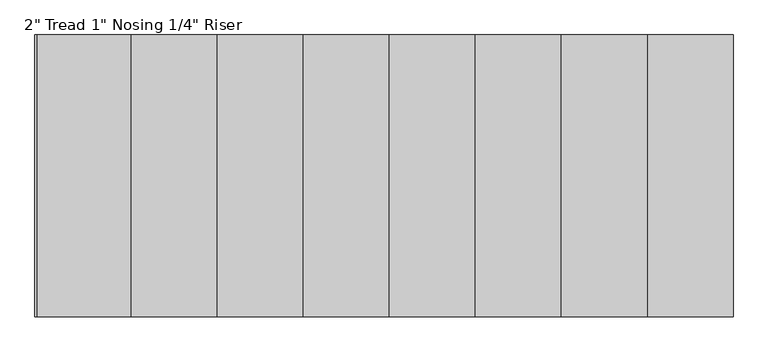
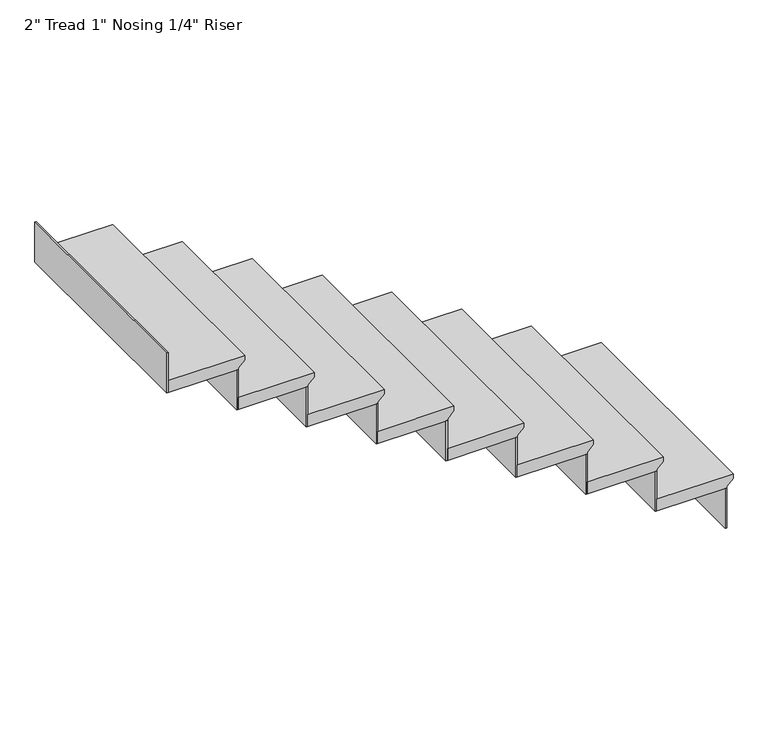
"""IFC4 building model written with IfcOpenShell, lengths in millimetres: stair flight geometry."""

from ifc_helpers import new_model, si_unit, frame, origin, place, context, project, spatial, polyline, outline, extrude, source, transform, mapped, element, save


def stair_flight_7c070f41(model_context):
    return source(origin(), model_context, "Body", "SweptSolid", [
        extrude(outline(polyline([(1998.1333333, -10706.2571222), (1998.1333333, -11011.0571222), (1947.3333333, -11011.0571222), (1947.3333333, -10731.6571222), (1953.6833333, -10731.6571222), (1979.0833333, -10706.2571222), (1998.1333333, -10706.2571222)])), frame((0.0, 5672.9776214, 0.0), z_axis=(0.0, 1.0, 0.0), x_axis=(0.0, 0.0, 1.0)), (0.0, 0.0, 1.0), 914.4),
        extrude(outline(polyline([(-10738.0071222, 6587.3776214), (-10731.6571222, 6587.3776214), (-10731.6571222, 5672.9776214), (-10738.0071222, 5672.9776214), (-10738.0071222, 6587.3776214)])), frame((0.0, 0.0, 1778.0), z_axis=(0.0, 0.0, 1.0), x_axis=(1.0, 0.0, 0.0)), (0.0, 0.0, 1.0), 169.3333333),
        extrude(outline(polyline([(-11017.4071222, 6587.3776214), (-11011.0571222, 6587.3776214), (-11011.0571222, 5672.9776214), (-11017.4071222, 5672.9776214), (-11017.4071222, 6587.3776214)])), frame((0.0, 0.0, 1947.3333333), z_axis=(0.0, 0.0, 1.0), x_axis=(1.0, 0.0, 0.0)), (0.0, 0.0, 1.0), 169.3333333),
        extrude(outline(polyline([(2167.4666667, -10985.6571222), (2167.4666667, -11290.4571222), (2116.6666667, -11290.4571222), (2116.6666667, -11011.0571222), (2123.0166667, -11011.0571222), (2148.4166667, -10985.6571222), (2167.4666667, -10985.6571222)])), frame((0.0, 5672.9776214, 0.0), z_axis=(0.0, 1.0, 0.0), x_axis=(0.0, 0.0, 1.0)), (0.0, 0.0, 1.0), 914.4),
        extrude(outline(polyline([(-11296.8071222, 6587.3776214), (-11290.4571222, 6587.3776214), (-11290.4571222, 5672.9776214), (-11296.8071222, 5672.9776214), (-11296.8071222, 6587.3776214)])), frame((0.0, 0.0, 2116.6666667), z_axis=(0.0, 0.0, 1.0), x_axis=(1.0, 0.0, 0.0)), (0.0, 0.0, 1.0), 169.3333333),
        extrude(outline(polyline([(2336.8, -11265.0571222), (2336.8, -11569.8571222), (2286.0, -11569.8571222), (2286.0, -11290.4571222), (2292.35, -11290.4571222), (2317.75, -11265.0571222), (2336.8, -11265.0571222)])), frame((0.0, 5672.9776214, 0.0), z_axis=(0.0, 1.0, 0.0), x_axis=(0.0, 0.0, 1.0)), (0.0, 0.0, 1.0), 914.4),
        extrude(outline(polyline([(-11576.2071222, 6587.3776214), (-11569.8571222, 6587.3776214), (-11569.8571222, 5672.9776214), (-11576.2071222, 5672.9776214), (-11576.2071222, 6587.3776214)])), frame((0.0, 0.0, 2286.0), z_axis=(0.0, 0.0, 1.0), x_axis=(1.0, 0.0, 0.0)), (0.0, 0.0, 1.0), 169.3333333),
        extrude(outline(polyline([(2506.1333333, -11544.4571222), (2506.1333333, -11849.2571222), (2455.3333333, -11849.2571222), (2455.3333333, -11569.8571222), (2461.6833333, -11569.8571222), (2487.0833333, -11544.4571222), (2506.1333333, -11544.4571222)])), frame((0.0, 5672.9776214, 0.0), z_axis=(0.0, 1.0, 0.0), x_axis=(0.0, 0.0, 1.0)), (0.0, 0.0, 1.0), 914.4),
        extrude(outline(polyline([(-11855.6071222, 6587.3776214), (-11849.2571222, 6587.3776214), (-11849.2571222, 5672.9776214), (-11855.6071222, 5672.9776214), (-11855.6071222, 6587.3776214)])), frame((0.0, 0.0, 2455.3333333), z_axis=(0.0, 0.0, 1.0), x_axis=(1.0, 0.0, 0.0)), (0.0, 0.0, 1.0), 169.3333333),
        extrude(outline(polyline([(2675.4666667, -11823.8571222), (2675.4666667, -12128.6571222), (2624.6666667, -12128.6571222), (2624.6666667, -11849.2571222), (2631.0166667, -11849.2571222), (2656.4166667, -11823.8571222), (2675.4666667, -11823.8571222)])), frame((0.0, 5672.9776214, 0.0), z_axis=(0.0, 1.0, 0.0), x_axis=(0.0, 0.0, 1.0)), (0.0, 0.0, 1.0), 914.4),
        extrude(outline(polyline([(-12135.0071222, 6587.3776214), (-12128.6571222, 6587.3776214), (-12128.6571222, 5672.9776214), (-12135.0071222, 5672.9776214), (-12135.0071222, 6587.3776214)])), frame((0.0, 0.0, 2624.6666667), z_axis=(0.0, 0.0, 1.0), x_axis=(1.0, 0.0, 0.0)), (0.0, 0.0, 1.0), 169.3333333),
        extrude(outline(polyline([(2844.8, -12103.2571222), (2844.8, -12408.0571222), (2794.0, -12408.0571222), (2794.0, -12128.6571222), (2800.35, -12128.6571222), (2825.75, -12103.2571222), (2844.8, -12103.2571222)])), frame((0.0, 5672.9776214, 0.0), z_axis=(0.0, 1.0, 0.0), x_axis=(0.0, 0.0, 1.0)), (0.0, 0.0, 1.0), 914.4),
        extrude(outline(polyline([(-12414.4071222, 6587.3776214), (-12408.0571222, 6587.3776214), (-12408.0571222, 5672.9776214), (-12414.4071222, 5672.9776214), (-12414.4071222, 6587.3776214)])), frame((0.0, 0.0, 2794.0), z_axis=(0.0, 0.0, 1.0), x_axis=(1.0, 0.0, 0.0)), (0.0, 0.0, 1.0), 169.3333333),
        extrude(outline(polyline([(3014.1333333, -12382.6571222), (3014.1333333, -12687.4571222), (2963.3333333, -12687.4571222), (2963.3333333, -12408.0571222), (2969.6833333, -12408.0571222), (2995.0833333, -12382.6571222), (3014.1333333, -12382.6571222)])), frame((0.0, 5672.9776214, 0.0), z_axis=(0.0, 1.0, 0.0), x_axis=(0.0, 0.0, 1.0)), (0.0, 0.0, 1.0), 914.4),
        extrude(outline(polyline([(-12693.8071222, 6587.3776214), (-12687.4571222, 6587.3776214), (-12687.4571222, 5672.9776214), (-12693.8071222, 5672.9776214), (-12693.8071222, 6587.3776214)])), frame((0.0, 0.0, 2963.3333333), z_axis=(0.0, 0.0, 1.0), x_axis=(1.0, 0.0, 0.0)), (0.0, 0.0, 1.0), 169.3333333),
        extrude(outline(polyline([(-12973.2071222, 6587.3776214), (-12966.8571222, 6587.3776214), (-12966.8571222, 5672.9776214), (-12973.2071222, 5672.9776214), (-12973.2071222, 6587.3776214)])), frame((0.0, 0.0, 3132.6666667), z_axis=(0.0, 0.0, 1.0), x_axis=(1.0, 0.0, 0.0)), (0.0, 0.0, 1.0), 169.3333333),
        extrude(outline(polyline([(3183.4666667, -12662.0571222), (3183.4666667, -12966.8571222), (3132.6666667, -12966.8571222), (3132.6666667, -12687.4571222), (3139.0166667, -12687.4571222), (3164.4166667, -12662.0571222), (3183.4666667, -12662.0571222)])), frame((0.0, 5672.9776214, 0.0), z_axis=(0.0, 1.0, 0.0), x_axis=(0.0, 0.0, 1.0)), (0.0, 0.0, 1.0), 914.4),
    ])


if __name__ == "__main__":
    model = new_model("IFC4")
    model_context = context("Model", 3, world=origin())
    ifc_project = project(units=[si_unit("LENGTHUNIT", "METRE", prefix="MILLI")], contexts=[model_context])
    site = spatial("IfcSite", under=ifc_project)
    building = spatial("IfcBuilding", under=site)
    placement = place(None, origin())
    stair_flight_shape = stair_flight_7c070f41(model_context)
    element("IfcStairFlight", 1, ObjectType="2\" Tread 1\" Nosing 1/4\" Riser", at=placement, inside=building, context=model_context, shape_type="MappedRepresentation", body=[
        mapped(stair_flight_shape, transform((0.0, 0.0, 0.0), x_axis=(1.0, 0.0, 0.0), y_axis=(0.0, 1.0, 0.0), z_axis=(0.0, 0.0, 1.0))),
    ])
    save(model, "model.ifc")
